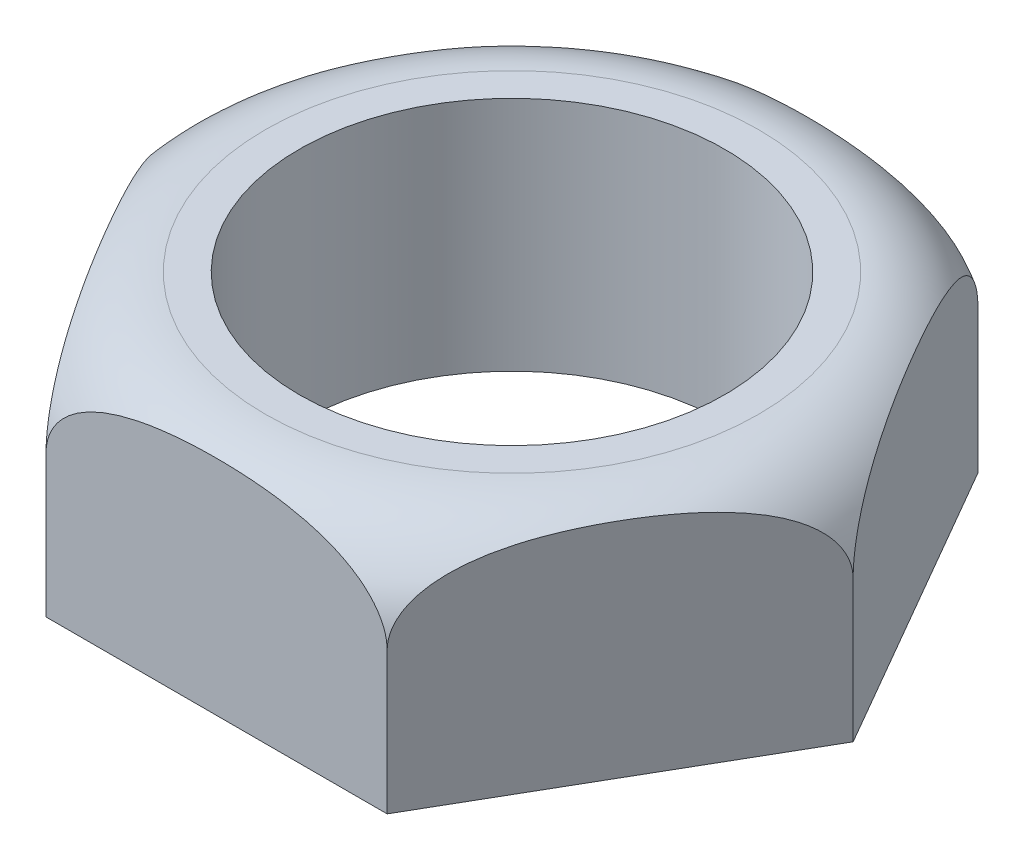
SolidWorks part; units mm, degrees
material "Plain Carbon Steel"
ref_plane "Front Plane" through (0, 0, 0) normal (0, 0, 1) x (1, 0, 0)
ref_plane "Top Plane" through (0, 0, 0) normal (0, 1, 0) x (1, 0, 0)
ref_plane "Right Plane" through (0, 0, 0) normal (1, 0, 0) x (0, 0, -1)
sketch "Hex Profile Sketch" plane through (0, 0, 0) normal (0, 1, 0) x (1, 0, 0)
  line L1 (14.4338, 0) -> (7.2169, 12.5)
  line L2 (7.2169, 12.5) -> (-7.2169, 12.5)
  line L3 (-7.2169, 12.5) -> (-14.4338, 0)
  line L4 (-14.4338, 0) -> (-7.2169, -12.5)
  line L5 (-7.2169, -12.5) -> (7.2169, -12.5)
  line L6 (7.2169, -12.5) -> (14.4338, 0)
  circle A0 centre (0, 0) radius 12.5 construction
  circle A1 centre (0, 0) radius 9
  dimension "D1" = 25
  dimension "D2" = 18
extrude "Hex Nut Body" add sketch "Hex Profile Sketch" along normal mid plane 10
sketch "Chamfer Profile Sketch" plane through (0, 0, 0) normal (0, 0, 1) x (1, 0, 0)
  line L0 (7.2169, 5) -> (14.4338, 5) construction
  line L1 (14.4338, 5) -> (14.4338, -5) construction
  line L2 (10.4338, 5) -> (14.4338, 5)
  line L3 (14.4338, 5) -> (14.4338, 1)
  line L4 (0, 0) -> (0, 21.3275) construction
  arc A0 (10.4338, 5) -> (14.4338, 1) centre (10.4338, 1) cw
  dimension "D1" = 4
revolve "Nut Chamfer Cut" cut sketch "Chamfer Profile Sketch" angle 360 about L4
